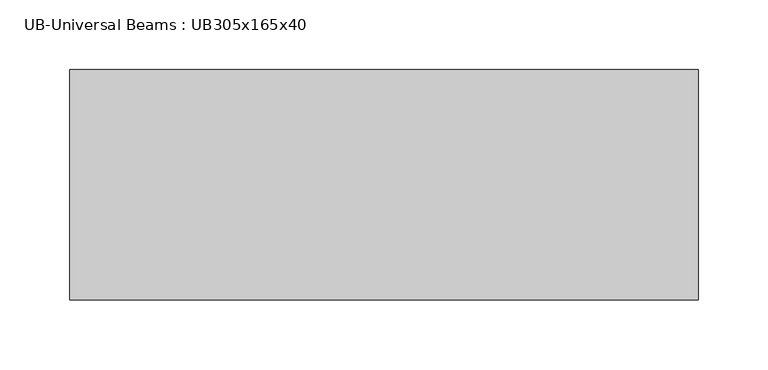
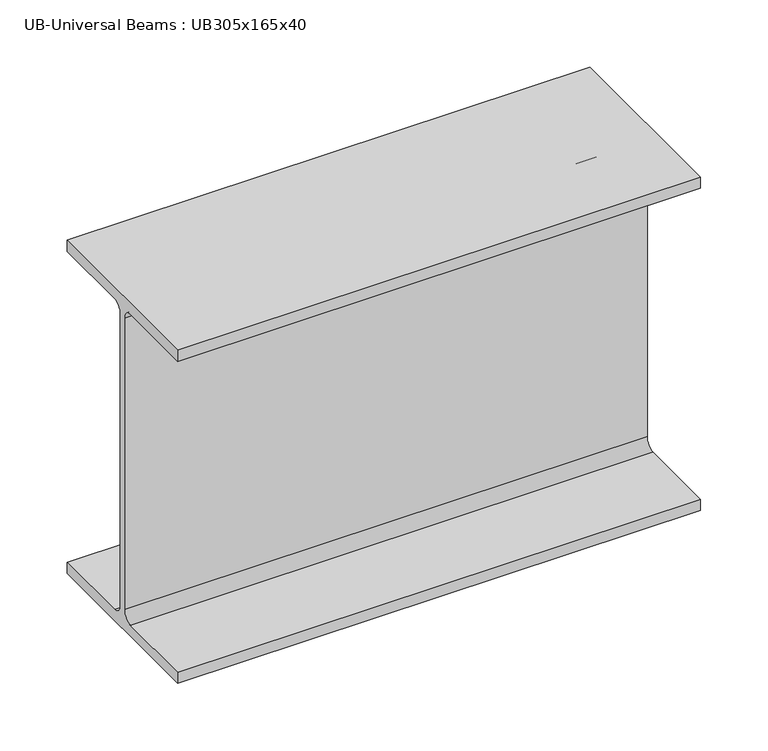
"""IFC4 building model written with IfcOpenShell, lengths in millimetres: beam geometry, UB-Universal Beams : UB305x165x40."""

from ifc_helpers import new_model, si_unit, point, frame, frame_2d, origin, place, context, project, spatial, polyline, circle_curve, trimmed, segment, composite_curve, outline, extrude, source, transform, mapped, element, save


def ub_universal_beams_ub305x165x40_d5ce0422(model_context):
    return source(origin(), model_context, "Body", "SweptSolid", [
        extrude(outline(composite_curve([segment(polyline([(82.5, -141.5), (82.5, -151.7), (-82.5, -151.7), (-82.5, -141.5), (-11.9, -141.5)]), True, "CONTINUOUS"), segment(trimmed(circle_curve(frame_2d((-11.9, -132.6)), 8.9), [point((-11.9, -141.5))], [point((-3.0, -132.6))], True, "CARTESIAN"), True, "CONTINUOUS"), segment(polyline([(-3.0, -132.6), (-3.0, 132.6)]), True, "CONTINUOUS"), segment(trimmed(circle_curve(frame_2d((-11.9, 132.6)), 8.9), [point((-3.0, 132.6))], [point((-11.9, 141.5))], True, "CARTESIAN"), True, "CONTINUOUS"), segment(polyline([(-11.9, 141.5), (-82.5, 141.5), (-82.5, 151.7), (82.5, 151.7), (82.5, 141.5), (11.9, 141.5)]), True, "CONTINUOUS"), segment(trimmed(circle_curve(frame_2d((11.9, 132.6)), 8.9), [point((11.9, 141.5))], [point((3.0, 132.6))], True, "CARTESIAN"), True, "CONTINUOUS"), segment(polyline([(3.0, 132.6), (3.0, -132.6)]), True, "CONTINUOUS"), segment(trimmed(circle_curve(frame_2d((11.9, -132.6)), 8.9), [point((3.0, -132.6))], [point((11.9, -141.5))], True, "CARTESIAN"), True, "CONTINUOUS"), segment(polyline([(11.9, -141.5), (82.5, -141.5)]), True, "CONTINUOUS")], self_intersect=False)), frame((-235.6, 0.0, 0.0), z_axis=(1.0, 0.0, 0.0), x_axis=(0.0, 1.0, 0.0)), (0.0, 0.0, 1.0), 449.9),
    ])


if __name__ == "__main__":
    model = new_model("IFC4")
    model_context = context("Model", 3, world=origin())
    ifc_project = project(units=[si_unit("LENGTHUNIT", "METRE", prefix="MILLI")], contexts=[model_context])
    site = spatial("IfcSite", under=ifc_project)
    building = spatial("IfcBuilding", under=site)
    placement = place(None, origin())
    ub_universal_beams_ub305x165x40_shape = ub_universal_beams_ub305x165x40_d5ce0422(model_context)
    element("IfcBeam", 1, ObjectType="UB-Universal Beams : UB305x165x40", at=placement, inside=building, context=model_context, shape_type="MappedRepresentation", body=[
        mapped(ub_universal_beams_ub305x165x40_shape, transform((0.0, 0.0, 0.0), x_axis=(1.0, 0.0, 0.0), y_axis=(0.0, 1.0, 0.0), z_axis=(0.0, 0.0, 1.0))),
    ])
    save(model, "model.ifc")

# Revit data of these elements
# Type "UB-Universal Beams : UB305x165x40"
#   Section Name Key = "UB305X165X40"
#   Width = 16.5 cm
#   Web Thickness = 0.6 cm
#   Web Fillet = 0.89 cm
#   Warping Constant = 164000.0 cm⁶
#   Torsional Moment of Inertia = 14.70 cm⁴
#   Section Area = 51.3 cm²
#   Plastic Modulus weak axis = 142.0 cm³
#   Plastic Modulus strong axis = 623.0 cm³
#   Nominal Weight = 40.2999 kgf/m
#   Moment of Inertia weak axis = 764.00 cm⁴
#   Moment of Inertia strong axis = 8503.00 cm⁴
#   Height = 30.34 cm
#   Flange Thickness = 1.02 cm
#   Elastic Modulus weak axis = 92.6 cm³
#   Elastic Modulus strong axis = 560.0 cm³
#   Centroid Vertical = 15.17 cm
#   Centroid Horizontal = 8.25 cm
#   Bolt Spacing = 9.0 cm
#   Length [instance default] = 1500 mm
#   Structural Material [instance default] = Metal - Steel 43-275
#   Type Comments = ""
#   Assembly Code = ""
# Element 1 (IfcBeam, "UB-Universal Beams : UB305x165x40")
#   Materials on its faces: "Metal - Steel 43-275"
# Materials
#   "Metal - Steel 43-275": class "Metal", colour RGB 247 247 247, transparency 0, Cost = 0
